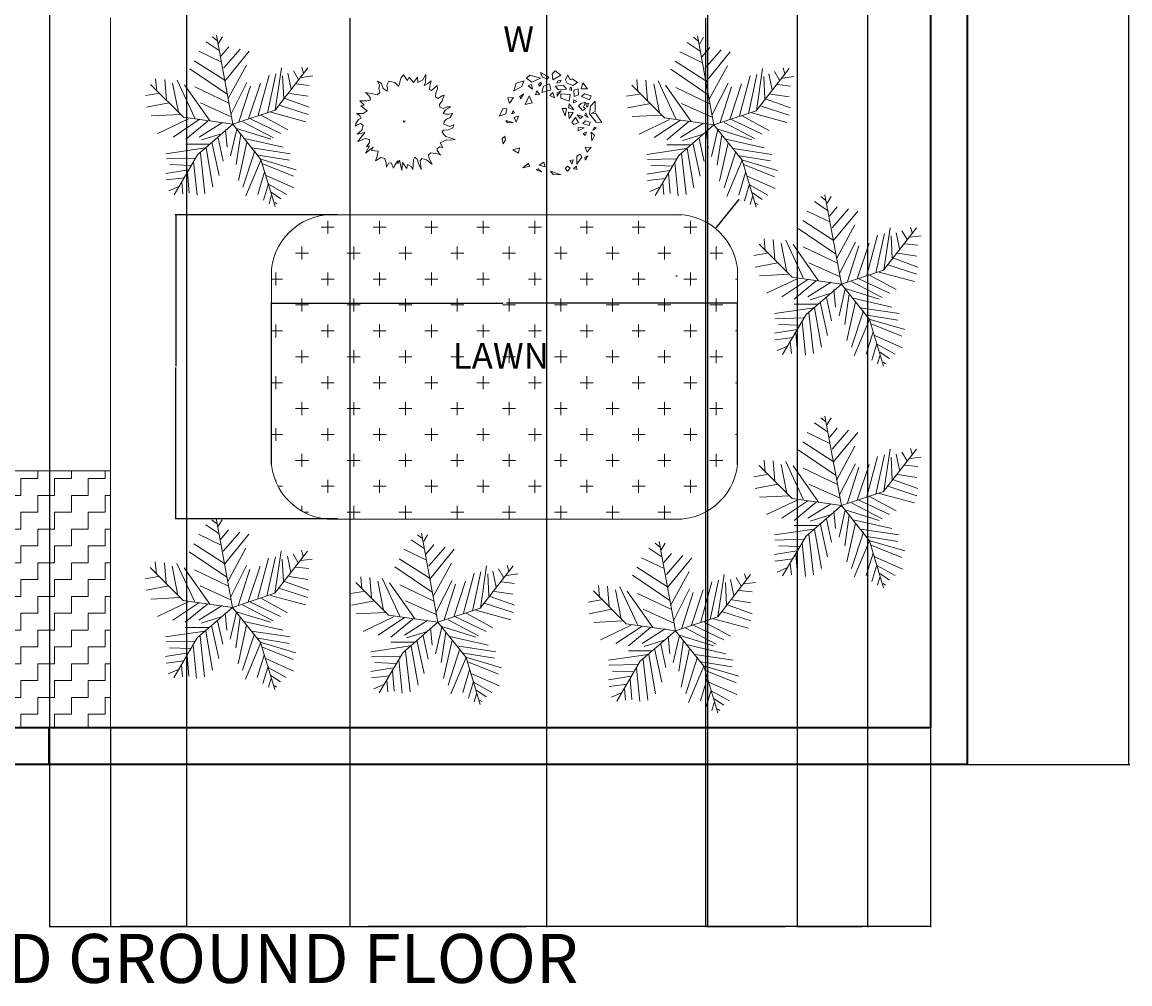
# Model space of a CAD drawing. Units: inches. Extents: x 2284 to 2815, y 1123 to 1948.
# Tile 3 of 6: x 2543 to 2814, y 1123 to 1358. Entities that reach past the tile are written whole.
import ezdxf

# ---------------------------------------------------------------- set-up
doc = ezdxf.new("R2010")
doc.units = ezdxf.units.IN
for name, color, linetype, lineweight in [('A-ANNO-DIMS', 2, 'Continuous', 18), ('A-ANNO-TITL', 30, 'Continuous', 35), ('A-AREA-IDEN', 30, 'Continuous', 18), ('A-WALL-PATT', 140, 'Continuous', 13), ('C-PVMT-PATT', 55, 'Continuous', 13), ('C-SITE-PVMT', 7, 'Continuous', 18), ('C-SITE-WALL', 7, 'Continuous', 35), ('L-FENC-GATE', 190, 'Continuous', 25), ('L-PLNT-BEDS', 90, 'Continuous', 18), ('L-PLNT-PATT', 40, 'Continuous', 13), ('TEXT', 30, 'Continuous', 18), ('TREE', 90, 'Continuous', 13)]:
    doc.layers.add(name, color=color, linetype=linetype, lineweight=lineweight)
doc.styles.get("Standard").update_dxf_attribs({"font": 'arial.ttf'})
doc.dimstyles.get("Standard").update_dxf_attribs({"dimtxt": 0.18, "dimasz": 0.18, "dimexe": 0.18, "dimexo": 0.0625, "dimgap": 0.09, "dimtad": 0, "dimtih": 1, "dimtoh": 1, "dimdec": 4, "dimzin": 0, "dimdsep": 46, "dimtxsty": 'Standard', "dimcen": 0.09, "dimadec": 0, "dimazin": 0, "dimtfac": 1, "dimtdec": 4, "dimtofl": 0, "dimtmove": 0, "dimatfit": 3, "dimfxl": 1, "dimtolj": 1, "dimtzin": 0, "dimarcsym": 0})

# ---------------------------------------------------------------- blocks, each defined once
blk = doc.blocks.new('*U9')
for points in [[(0, 60.64), (-3.051, 56.238), (-4.196, 52.815), (-5.34, 47.925), (-6.103, 45.969), (-11.062, 50.859), (-18.691, 52.326), (-20.98, 47.436), (-20.217, 43.524), (-20.598, 39.611), (-25.939, 43.035), (-27.846, 49.392), (-33.186, 52.326), (-30.516, 47.436), (-31.279, 43.035), (-30.135, 38.144), (-33.568, 35.21), (-40.815, 36.677), (-49.208, 38.144), (-46.919, 36.677), (-42.341, 31.787), (-42.341, 28.364), (-46.537, 27.386), (-55.692, 27.386), (-49.97, 22.006), (-54.548, 21.028), (-46.156, 14.671), (-51.496, 11.248), (-59.888, 11.248), (-55.692, 8.803), (-53.785, 5.38), (-57.218, 3.423), (-60.651, -1.467), (-61.033, -4.89), (-59.125, -3.423), (-54.548, -1.467), (-51.496, -4.401), (-53.022, -10.269), (-59.125, -15.16), (-49.208, -13.204), (-58.362, -24.451), (-48.445, -21.028), (-43.486, -22.495), (-43.104, -25.918), (-47.3, -31.298), (-43.104, -30.32), (-48.445, -39.611), (-38.527, -31.787), (-40.815, -36.188), (-32.423, -37.166), (-33.568, -43.523), (-35.475, -49.392), (-28.609, -44.99), (-23.65, -46.457), (-22.124, -51.837), (-21.743, -57.705), (-19.073, -52.326), (-15.639, -51.837), (-12.588, -58.683), (-11.062, -54.771), (-6.866, -49.392), (-6.866, -53.304), (-4.959, -48.414), (-1.907, -61.617), (-1.144, -51.348), (4.578, -59.172), (5.341, -54.282), (9.918, -56.727), (12.207, -60.639), (12.97, -47.925), (14.877, -44.501), (17.547, -47.436), (19.455, -52.815), (22.888, -60.639), (21.743, -49.392), (23.65, -46.457), (29.754, -47.925), (35.094, -52.326), (37.001, -53.793), (33.187, -46.457), (32.042, -41.567), (35.094, -39.122), (43.868, -40.589), (47.682, -42.056), (43.105, -36.188), (43.105, -33.743), (46.538, -31.298), (50.352, -32.765), (46.919, -26.407), (55.693, -22.495), (60.652, -22.984), (66.374, -22.006), (59.889, -20.05), (54.167, -18.094), (51.878, -15.649), (49.589, -12.225), (51.497, -10.269), (57.981, -9.78), (63.322, -7.335), (64.466, -2.934)], [(64.848, -2.934), (59.507, -5.379), (56.456, -4.401), (51.878, -2.445), (52.26, 0.978), (55.311, 3.912), (59.889, 5.869), (62.94, 11.248), (58.363, 10.27), (54.548, 10.27), (51.115, 11.248), (53.785, 15.649), (57.981, 18.094), (60.652, 19.561), (56.074, 19.561), (51.115, 17.605), (46.538, 19.072), (46.156, 22.496), (49.589, 27.386), (52.26, 34.721), (49.589, 33.743), (44.249, 30.32), (41.197, 32.276), (41.579, 37.655), (43.868, 42.546), (43.105, 46.947), (40.053, 44.013), (36.238, 40.589), (33.568, 42.057), (33.95, 45.969), (35.476, 52.815), (31.28, 49.392), (26.702, 46.947), (28.228, 50.859), (28.609, 61.129), (24.795, 54.282), (18.692, 50.859), (17.929, 57.706), (12.97, 50.859), (7.248, 57.706), (5.341, 53.304), (0, 60.64)]]:
    blk.add_lwpolyline(points)
blk.add_lwpolyline([(0.382, 1.956), (0, 0), (1.907, 0.489), (2.289, 1.467)], close=True)
blk = doc.blocks.new('*U6')
for p, q in [((0, 0), (-10.5, 57)), ((-8.737, 47.138), (-17.069, 52.711)), ((-10.186, 53.64), (-13.084, 55.962)), ((-9.099, 51.782), (-6.563, 55.962)), ((-7.288, 39.707), (-21.778, 46.673)), ((-7.65, 43.423), (-2.578, 49.46)), ((-5.839, 35.992), (4.667, 48.067)), ((-5.114, 27.632), (10.463, 46.673)), ((-3.665, 19.273), (-27.574, 35.527)), ((-5.114, 28.097), (-24.676, 40.636)), ((-2.941, 16.486), (8.652, 37.85)), ((27, 9), (48, 36)), ((27.127, 9.056), (31.112, 35.992)), ((44.153, 36.456), (45.239, 32.741)), ((-48.585, 21.131), (-49.309, 29.026)), ((-43.513, 28.561), (-42.427, 15.558)), ((16.259, 5.805), (23.142, 31.348)), ((22.055, 7.198), (27.489, 32.277)), ((31.836, 30.883), (32.561, 16.486)), ((35.096, 32.741), (37.27, 22.524)), ((38.719, 34.134), (41.979, 28.561)), ((43.791, 29.954), (51.036, 30.883)), ((-31.5, 4.5), (-52.5, 25.5)), ((-38.442, 26.239), (-34.819, 7.663)), ((-35.544, 28.097), (-24.314, 3.947)), ((-14.533, 2.09), (-30.834, 25.31)), ((-24.314, 23.917), (-2.941, 13.7)), ((-1.129, 6.734), (9.014, 26.704)), ((3.942, 1.625), (11.187, 24.381)), ((10.101, 3.483), (17.708, 26.239)), ((40.53, 25.775), (48.862, 24.846)), ((-47.498, 19.737), (-55.83, 18.344)), ((33.285, 16.486), (48.862, 10.913)), ((36.183, 19.737), (48.137, 17.88)), ((-40.615, 13.7), (-55.105, 10.913)), ((-20.691, 13.7), (-1.129, 4.876)), ((0, 0), (27, 9)), ((24.229, 7.663), (46.688, 1.625)), ((29.662, 12.307), (48.137, 6.269)), ((-33.37, 6.269), (-52.207, 5.34)), ((-28.299, 3.483), (-47.86, -5.805)), ((-21.416, 3.018), (-38.079, -8.128)), ((0, 0), (-31.5, 4.5)), ((-15.982, 2.09), (-30.11, -9.521)), ((0, 0), (-22.5, -19.5)), ((-6.563, 1.161), (-21.416, -8.128)), ((0, 0), (18, -22.5)), ((6.478, 1.625), (26.04, -8.592)), ((11.187, 3.483), (30.749, -5.805)), ((18.07, 5.805), (35.096, -3.483)), ((-6.563, -5.805), (-19.967, -9.985)), ((-4.752, -3.483), (-3.665, -14.629)), ((2.493, -3.019), (-1.491, -20.202)), ((1.769, -2.555), (24.229, -9.521)), ((5.029, -6.27), (2.131, -25.775)), ((-15.257, -12.772), (-30.11, -12.772)), ((-13.446, -11.378), (-8.737, -32.741)), ((-9.461, -8.592), (-6.201, -23.453)), ((9.014, -11.378), (3.58, -35.992)), ((7.565, -9.056), (32.198, -14.629)), ((-17.431, -15.094), (-42.789, -18.809)), ((-22.5, -19.5), (-37.5, -45)), ((-20.691, -18.345), (-17.793, -44.352)), ((-17.069, -15.094), (-12.721, -40.172)), ((14.085, -16.951), (6.478, -40.172)), ((12.274, -15.094), (36.907, -18.809)), ((16.259, -19.738), (36.183, -22.989)), ((-24.314, -21.596), (-42.427, -22.06)), ((-26.849, -26.24), (-40.253, -25.775)), ((-25.038, -23.918), (-22.865, -45.281)), ((18.07, -22.524), (8.289, -45.745)), ((18, -22.5), (27, -52.5)), ((18.433, -22.524), (40.53, -29.026)), ((19.157, -25.311), (38.719, -33.206)), ((-28.299, -29.026), (-42.789, -31.348)), ((-30.834, -34.135), (-42.427, -35.528)), ((-29.023, -30.884), (-27.936, -43.887)), ((20.244, -30.419), (15.897, -44.816)), ((21.331, -32.741), (39.081, -40.636)), ((-34.457, -39.708), (-40.978, -42.494)), ((-32.646, -36.921), (-31.921, -44.352)), ((22.78, -37.85), (19.519, -48.532)), ((22.78, -38.314), (34.372, -44.816)), ((24.591, -45.745), (23.142, -50.854)), ((24.591, -43.423), (30.749, -47.603)), ((26.764, -49.925), (28.213, -50.854))]:
    blk.add_line(p, q)
blk = doc.blocks.new('*U10')
for points in [[(-4.43, 11.05), (-5.18, 10.36), (-3.96, 9.49), (-2.07, 10.36)], [(-2, 11.66), (-1.6, 10.62), (-0.52, 10.1), (-0.18, 10.62), (-0.79, 10.96)], [(1.24, 12), (0.56, 11.31), (0.76, 10.01), (2.52, 11.05)], [(4.14, 11.14), (3.6, 10.01), (4, 9.23), (5.22, 8.71), (6.3, 9.41), (5.08, 10.19), (4.61, 10.01)], [(-5.78, 9.75), (-7.54, 9.23), (-8.01, 7.5), (-6.26, 8.45)], [(-4.84, 8.63), (-3.83, 7.85), (-4.03, 8.97)], [(-2.88, 7.5), (-3.15, 6.64), (-2.27, 6.72)], [(-1.94, 9.49), (-2.48, 8.97), (-2.27, 8.54), (-1.8, 9.06)], [(0.02, 9.06), (-1.33, 8.54), (-1.73, 7.16), (0.29, 7.76)], [(1.37, 8.54), (3.13, 8.8), (3.8, 7.85), (1.91, 7.76)], [(2.59, 9.93), (1.84, 9.75), (1.64, 9.23), (2.32, 9.41)], [(1.71, 6.29), (1.71, 7.07), (2.65, 7.5), (2.11, 6.9)], [(4.61, 8.28), (4.54, 7.76), (4.95, 7.59), (4.95, 8.28)], [(6.43, 7.94), (5.49, 7.68), (5.56, 6.21), (6.5, 6.64)], [(7.45, 9.32), (7.11, 7.94), (8.52, 7.94)], [(-8.14, 6.03), (-9.36, 5.95), (-9.02, 4.73)], [(-5.78, 6.81), (-6.66, 6.21), (-6.52, 5.69)], [(-4.57, 6.38), (-5.45, 4.47), (-3.89, 4.82)], [(0.76, 7.16), (0.09, 6.46), (1.1, 5.95)], [(2.52, 6.81), (2.52, 5.86), (4.41, 5.17), (4.61, 6.72)], [(5.49, 5.51), (5.42, 4.82), (6.16, 5.08)], [(8.12, 4.99), (7.11, 4.65), (6.5, 4.13), (7.38, 3.09), (8.12, 3.52), (7.65, 3.87)], [(7.85, 6.81), (7.18, 6.21), (9, 5.51), (9.33, 6.38)], [(10.28, 5.17), (9.2, 4.04), (9, 2.31), (10.48, 0.49), (11.76, 0.41), (10.35, 2.48), (9.33, 2.4), (10.28, 2.83)], [(-11.32, 1.79), (-9.83, 2.31), (-9.63, 3.44), (-10.44, 3.52)], [(-8.21, 3.09), (-8.48, 2.31), (-7.87, 2.57)], [(3.53, 1.88), (2.86, 3.52), (3.8, 3.52)], [(4.41, 4.56), (4.27, 3.7), (5.49, 3.26)], [(4.27, 2.74), (5.29, 2.66), (4.41, 1.27)], [(8.19, 2.57), (7.92, 2.05), (8.66, 1.53)], [(8.73, 4.73), (8.19, 4.56), (8.39, 3.87), (8.59, 4.04)], [(-8.21, 0.41), (-9.43, 0.32), (-9.83, 0.84)], [(-7, 1.79), (-7.94, 1.53), (-7.47, 0.49)], [(5.83, 1.53), (5.02, 0.41), (5.49, -0.02), (6.5, 0.41)], [(7.51, 1.71), (6.91, 1.27), (6.23, 2.14)], [(8.12, 0.75), (7.51, 0.15), (8.93, -0.28), (9.13, 0.49)], [(7.78, -0.8), (6.43, -1.5), (6.43, -0.72)], [(8.32, -1.75), (7.98, -2.53), (7.58, -2.1)], [(9.33, -1.75), (9.54, -3.74), (10.14, -2.53)], [(10.08, -0.63), (9.74, -1.32), (10.48, -0.89)], [(-10.03, -2.71), (-10.64, -3.31), (-10.44, -4.44), (-9.9, -3.49)], [(-8.28, -5.73), (-6.79, -5.3), (-7, -6.51)], [(6.1, -8.94), (6.16, -7.21), (6.91, -6.69), (7.24, -7.38)], [(8.05, -8.07), (8.59, -7.12), (7.92, -7.55)], [(9.33, -5.13), (8.46, -6.25), (7.98, -5.22)], [(-4.84, -8.85), (-4.43, -9.45), (-5.99, -9.8)], [(-2.34, -9.2), (-1.26, -8.5), (-0.99, -9.54)], [(4.07, -9.45), (3.53, -9.97), (4.07, -10.58), (4.61, -9.89)], [(5.29, -7.98), (4.61, -8.16), (5.02, -8.94)], [(6.03, -9.45), (5.42, -9.97), (6.16, -10.15)], [(-2.54, -10.06), (-3.02, -10.23), (-1.8, -10.67)], [(0.22, -10.58), (0.83, -11.27), (2.59, -11.36)]]:
    blk.add_lwpolyline(points, close=True)
blk = doc.blocks.new('*D21')
at = {"layer": 'A-ANNO-DIMS', "color": 0, "lineweight": -2, "transparency": 16777216}
for p, q in [((2774.62, 1908.4), (2814.43, 1908.4)), ((2814.25, 1908.22), (2814.25, 1542.59)), ((2814.25, 1176.58), (2814.25, 1542.22)), ((2774.62, 1176.4), (2814.43, 1176.4))]:
    blk.add_line(p, q, dxfattribs=at)
at = {"layer": 'A-ANNO-DIMS', "color": 0, "transparency": 16777216}
for points in [[(2814.22, 1908.22), (2814.28, 1908.22), (2814.25, 1908.4)], [(2814.22, 1176.58), (2814.28, 1176.58), (2814.25, 1176.4)]]:
    blk.add_solid(points, dxfattribs=at)
at = {"layer": 'Defpoints', "color": 0, "transparency": 16777216}
for p in [(2774.55, 1908.4), (2814.25, 1908.4), (2774.55, 1176.4)]:
    blk.add_point(p, dxfattribs=at)
at = {"layer": 'A-ANNO-DIMS', "color": 0, "transparency": 16777216, "insert": (2814.25, 1542.4), "char_height": 0.18, "attachment_point": 5}
blk.add_mtext('\\A1;732', dxfattribs=at)
blk = doc.blocks.new('*D41')
at = {"layer": 'A-ANNO-DIMS', "color": 0, "lineweight": -2, "transparency": 16777216}
for p, q in [((2564.55, 1185.34), (2564.55, 1136.52)), ((2765.55, 1185.34), (2765.55, 1136.52)), ((2564.73, 1136.7), (2664.78, 1136.7)), ((2765.37, 1136.7), (2665.33, 1136.7))]:
    blk.add_line(p, q, dxfattribs=at)
at = {"layer": 'A-ANNO-DIMS', "color": 0, "transparency": 16777216}
for points in [[(2564.73, 1136.73), (2564.73, 1136.67), (2564.55, 1136.7)], [(2765.37, 1136.73), (2765.37, 1136.67), (2765.55, 1136.7)]]:
    blk.add_solid(points, dxfattribs=at)
at = {"layer": 'Defpoints', "color": 0, "transparency": 16777216}
for p in [(2564.55, 1185.4), (2765.55, 1185.4), (2765.55, 1136.7)]:
    blk.add_point(p, dxfattribs=at)
at = {"layer": 'A-ANNO-DIMS', "color": 0, "transparency": 16777216, "insert": (2665.05, 1136.7), "char_height": 0.18, "attachment_point": 5}
blk.add_mtext('\\A1;201', dxfattribs=at)
blk = doc.blocks.new('*D42')
at = {"layer": 'A-ANNO-DIMS', "color": 0, "lineweight": -2, "transparency": 16777216}
for p, q in [((2623.18, 1359.34), (2623.18, 1136.52)), ((2710.41, 1359.34), (2710.41, 1136.52)), ((2623.36, 1136.7), (2666.4, 1136.7)), ((2710.23, 1136.7), (2667.19, 1136.7))]:
    blk.add_line(p, q, dxfattribs=at)
at = {"layer": 'A-ANNO-DIMS', "color": 0, "transparency": 16777216}
for points in [[(2623.36, 1136.73), (2623.36, 1136.67), (2623.18, 1136.7)], [(2710.23, 1136.73), (2710.23, 1136.67), (2710.41, 1136.7)]]:
    blk.add_solid(points, dxfattribs=at)
at = {"layer": 'Defpoints', "color": 0, "transparency": 16777216}
for p in [(2623.18, 1359.4), (2710.41, 1359.4), (2710.41, 1136.7)]:
    blk.add_point(p, dxfattribs=at)
at = {"layer": 'A-ANNO-DIMS', "color": 0, "transparency": 16777216, "insert": (2666.79, 1136.7), "char_height": 0.18, "attachment_point": 5}
blk.add_mtext('\\A1;87.23', dxfattribs=at)
blk = doc.blocks.new('*D44')
at = {"layer": 'A-ANNO-DIMS', "color": 0, "lineweight": -2, "transparency": 16777216}
for p, q in [((2583.19, 1836.34), (2583.19, 1136.52)), ((2671.4, 1836.34), (2671.4, 1136.52)), ((2583.37, 1136.7), (2626.92, 1136.7)), ((2671.22, 1136.7), (2627.67, 1136.7))]:
    blk.add_line(p, q, dxfattribs=at)
at = {"layer": 'A-ANNO-DIMS', "color": 0, "transparency": 16777216}
for points in [[(2583.37, 1136.73), (2583.37, 1136.67), (2583.19, 1136.7)], [(2671.22, 1136.73), (2671.22, 1136.67), (2671.4, 1136.7)]]:
    blk.add_solid(points, dxfattribs=at)
at = {"layer": 'Defpoints', "color": 0, "transparency": 16777216}
for p in [(2583.19, 1836.4), (2671.4, 1836.4), (2671.4, 1136.7)]:
    blk.add_point(p, dxfattribs=at)
at = {"layer": 'A-ANNO-DIMS', "color": 0, "transparency": 16777216, "insert": (2627.29, 1136.7), "char_height": 0.18, "attachment_point": 5}
blk.add_mtext('\\A1;88.21', dxfattribs=at)
blk = doc.blocks.new('*D45')
at = {"layer": 'A-ANNO-DIMS', "color": 0, "lineweight": -2, "transparency": 16777216}
for p, q in [((2549.55, 1836.34), (2549.55, 1136.52)), ((2583.19, 1836.34), (2583.19, 1136.52)), ((2549.73, 1136.7), (2565.91, 1136.7)), ((2583.01, 1136.7), (2566.84, 1136.7))]:
    blk.add_line(p, q, dxfattribs=at)
at = {"layer": 'A-ANNO-DIMS', "color": 0, "transparency": 16777216}
for points in [[(2549.73, 1136.73), (2549.73, 1136.67), (2549.55, 1136.7)], [(2583.01, 1136.73), (2583.01, 1136.67), (2583.19, 1136.7)]]:
    blk.add_solid(points, dxfattribs=at)
at = {"layer": 'Defpoints', "color": 0, "transparency": 16777216}
for p in [(2549.55, 1836.4), (2583.19, 1836.4), (2583.19, 1136.7)]:
    blk.add_point(p, dxfattribs=at)
at = {"layer": 'A-ANNO-DIMS', "color": 0, "transparency": 16777216, "insert": (2566.37, 1136.7), "char_height": 0.18, "attachment_point": 5}
blk.add_mtext('\\A1;33.635', dxfattribs=at)
blk = doc.blocks.new('*D49')
at = {"layer": 'A-ANNO-DIMS', "color": 0, "lineweight": -2, "transparency": 16777216}
for p, q in [((2732.88, 1524.34), (2732.88, 1136.52)), ((2765.55, 1524.34), (2765.55, 1136.52)), ((2733.06, 1136.7), (2748.82, 1136.7)), ((2765.37, 1136.7), (2749.61, 1136.7))]:
    blk.add_line(p, q, dxfattribs=at)
at = {"layer": 'A-ANNO-DIMS', "color": 0, "transparency": 16777216}
for points in [[(2733.06, 1136.73), (2733.06, 1136.67), (2732.88, 1136.7)], [(2765.37, 1136.73), (2765.37, 1136.67), (2765.55, 1136.7)]]:
    blk.add_solid(points, dxfattribs=at)
at = {"layer": 'Defpoints', "color": 0, "transparency": 16777216}
for p in [(2732.88, 1524.4), (2765.55, 1524.4), (2765.55, 1136.7)]:
    blk.add_point(p, dxfattribs=at)
at = {"layer": 'A-ANNO-DIMS', "color": 0, "transparency": 16777216, "insert": (2749.21, 1136.7), "char_height": 0.18, "attachment_point": 5}
blk.add_mtext('\\A1;32.68', dxfattribs=at)
blk = doc.blocks.new('*D51')
at = {"layer": 'A-ANNO-DIMS', "color": 0, "lineweight": -2, "transparency": 16777216}
for p, q in [((2710.87, 1388.93), (2710.87, 1136.52)), ((2750.11, 1388.93), (2750.11, 1136.52)), ((2711.05, 1136.7), (2730.03, 1136.7)), ((2749.93, 1136.7), (2730.95, 1136.7))]:
    blk.add_line(p, q, dxfattribs=at)
at = {"layer": 'A-ANNO-DIMS', "color": 0, "transparency": 16777216}
for points in [[(2711.05, 1136.73), (2711.05, 1136.67), (2710.87, 1136.7)], [(2749.93, 1136.73), (2749.93, 1136.67), (2750.11, 1136.7)]]:
    blk.add_solid(points, dxfattribs=at)
at = {"layer": 'Defpoints', "color": 0, "transparency": 16777216}
for p in [(2710.87, 1389), (2750.11, 1389), (2750.11, 1136.7)]:
    blk.add_point(p, dxfattribs=at)
at = {"layer": 'A-ANNO-DIMS', "color": 0, "transparency": 16777216, "insert": (2730.49, 1136.7), "char_height": 0.18, "attachment_point": 5}
blk.add_mtext('\\A1;39.234', dxfattribs=at)
blk = doc.blocks.new('*D57')
at = {"layer": 'A-ANNO-DIMS', "color": 0, "lineweight": -2, "transparency": 16777216}
for p, q in [((2604.02, 1249.87), (2604.02, 1289.69)), ((2604.2, 1289.51), (2660.68, 1289.51)), ((2718.06, 1289.51), (2661.59, 1289.51)), ((2718.24, 1249.87), (2718.24, 1289.69))]:
    blk.add_line(p, q, dxfattribs=at)
at = {"layer": 'A-ANNO-DIMS', "color": 0, "transparency": 16777216}
for points in [[(2604.2, 1289.54), (2604.2, 1289.48), (2604.02, 1289.51)], [(2718.06, 1289.54), (2718.06, 1289.48), (2718.24, 1289.51)]]:
    blk.add_solid(points, dxfattribs=at)
at = {"layer": 'Defpoints', "color": 0, "transparency": 16777216}
for p in [(2718.24, 1289.51), (2604.02, 1249.81), (2718.24, 1249.81)]:
    blk.add_point(p, dxfattribs=at)
at = {"layer": 'A-ANNO-DIMS', "color": 0, "transparency": 16777216, "insert": (2661.13, 1289.51), "char_height": 0.18, "attachment_point": 5}
blk.add_mtext('\\A1;114.22', dxfattribs=at)
blk = doc.blocks.new('*D58')
at = {"layer": 'A-ANNO-DIMS', "color": 0, "lineweight": -2, "transparency": 16777216}
for p, q in [((2620.16, 1311.15), (2580.34, 1311.15)), ((2580.52, 1310.97), (2580.52, 1274.05)), ((2580.52, 1236.77), (2580.52, 1273.69)), ((2620.16, 1236.59), (2580.34, 1236.59))]:
    blk.add_line(p, q, dxfattribs=at)
at = {"layer": 'A-ANNO-DIMS', "color": 0, "transparency": 16777216}
for points in [[(2580.49, 1310.97), (2580.55, 1310.97), (2580.52, 1311.15)], [(2580.49, 1236.77), (2580.55, 1236.77), (2580.52, 1236.59)]]:
    blk.add_solid(points, dxfattribs=at)
at = {"layer": 'Defpoints', "color": 0, "transparency": 16777216}
for p in [(2580.52, 1311.15), (2620.22, 1311.15), (2620.22, 1236.59)]:
    blk.add_point(p, dxfattribs=at)
at = {"layer": 'A-ANNO-DIMS', "color": 0, "transparency": 16777216, "insert": (2580.52, 1273.87), "char_height": 0.18, "attachment_point": 5}
blk.add_mtext('\\A1;74.56', dxfattribs=at)
blk = doc.blocks.new('*D59')
at = {"layer": 'A-ANNO-DIMS', "color": 0, "lineweight": -2, "transparency": 16777216}
for p, q in [((2718.52, 1314.79), (2712.94, 1307.96)), ((2718.7, 1314.79), (2718.52, 1314.79)), ((2703.25, 1296.21), (2703.43, 1296.21)), ((2703.34, 1296.12), (2703.34, 1296.3))]:
    blk.add_line(p, q, dxfattribs=at)
at = {"layer": 'A-ANNO-DIMS', "color": 0, "transparency": 16777216}
blk.add_solid([(2712.92, 1307.98), (2712.96, 1307.94), (2712.83, 1307.82)], dxfattribs=at)
at = {"layer": 'Defpoints', "color": 0, "transparency": 16777216}
for p in [(2712.83, 1307.82), (2703.34, 1296.21)]:
    blk.add_point(p, dxfattribs=at)
at = {"layer": 'A-ANNO-DIMS', "color": 0, "transparency": 16777216, "insert": (2719.44, 1314.79), "char_height": 0.18, "attachment_point": 5}
blk.add_mtext('\\A1;4X R14.997', dxfattribs=at)

msp = doc.modelspace()

# ---------------------------------------------------------------- hatches: boundary and pattern name
at = {"layer": 'A-WALL-PATT'}
h = msp.add_hatch(dxfattribs=at)
h.set_pattern_fill('AR-SAND', color=256, scale=8.5)
h.paths.add_polyline_path([(2339.554, 1899.404), (2375.554, 1899.404), (2765.554, 1899.404), (2765.554, 1185.404), (2549.3222, 1185.404), (2549.3222, 1176.404), (2774.554, 1176.404), (2774.554, 1908.404), (2330.554, 1908.404), (2330.554, 1176.404), (2349.4276, 1176.404), (2349.4276, 1185.404), (2339.554, 1185.404)])
h.paths.add_polyline_path([(2710.054, 1899.404), (2701.054, 1899.404), (2701.054, 1889.8374), (2710.054, 1889.8374)], flags=17)
at = {"layer": 'C-PVMT-PATT'}
h = msp.add_hatch(dxfattribs=at)
h.set_pattern_fill('ZIGZAG', color=256, scale=1.3)
h.set_pattern_definition([(0, (0, 0), (4.1275, 4.1275), [4.1275, -4.1275]), (90, (4.1275, 0), (-4.1275, 4.1275), [4.1275, -4.1275])])
h.paths.add_polyline_path([(2564.554, 1248.417), (2339.554, 1248.417), (2339.554, 1185.404), (2564.554, 1185.404)])
at = {"layer": 'L-PLNT-PATT'}
h = msp.add_hatch(dxfattribs=at)
h.set_pattern_fill('CROSS', color=256)
h.paths.add_polyline_path([(2718.2406, 1297.9246, 0.35632969), (2704.6415, 1311.1466), (2617.6203, 1311.1466, 0.35632969), (2604.0213, 1297.9246), (2604.0213, 1249.8094, 0.35632969), (2617.6203, 1236.5875), (2704.6415, 1236.5875, 0.35632969), (2718.2406, 1249.8094)])

# ---------------------------------------------------------------- linework, layer by layer
at = {"layer": 'C-SITE-PVMT'}
for p, q in [((2564.554, 1359.404), (2564.554, 1185.404)), ((2339.554, 1248.417), (2564.554, 1248.417))]:
    msp.add_line(p, q, dxfattribs=at)
at = {"layer": 'C-SITE-WALL'}
for p, q in [((2774.554, 1908.404), (2774.554, 1176.404)), ((2765.554, 1899.404), (2765.554, 1185.404)), ((2765.554, 1185.404), (2339.554, 1185.404)), ((2774.554, 1176.404), (2330.554, 1176.404))]:
    msp.add_line(p, q, dxfattribs=at)
at = {"layer": 'L-FENC-GATE'}
msp.add_line((2549.3222, 1185.404), (2549.3222, 1176.404), dxfattribs=at)
at = {"layer": 'L-PLNT-BEDS'}
for points in [[(2617.6203, 1311.1466), (2704.6415, 1311.1466)], [(2604.0213, 1249.8094), (2604.0213, 1297.9246)], [(2718.2406, 1297.9246), (2718.2406, 1249.8094)], [(2704.6415, 1236.5875), (2617.6203, 1236.5875)]]:
    msp.add_lwpolyline(points, dxfattribs=at)
for centre, start, end in [((2618.9194, 1296.206), 85.030532, 173.41944), ((2703.3424, 1296.206), 6.58056, 94.969468), ((2618.9194, 1251.5281), 186.58056, 274.969468), ((2703.3424, 1251.5281), 265.030532, 353.41944)]:
    msp.add_arc(centre, 14.997, start, end, dxfattribs=at)

# ---------------------------------------------------------------- block references
at = {"layer": 'TREE'}
for name, p, xscale, yscale, zscale in [('*U6', (2594.5131, 1333.3351), 0.383737482457664, 0.383737482457664, 0.383737482457664), ('*U6', (2712.4723, 1333.1807), 0.383737482457664, 0.383737482457664, 0.383737482457664), ('*U9', (2636.3223, 1333.8468), 0.1916033270346016, 0.1916033270346016, 0.1916033270346016), ('*U10', (2672.1718, 1333.3502), 1.090243299178313, 1.090243299178313, 1.090243299178313), ('*U6', (2743.717, 1294.1583), 0.383737482457664, 0.383737482457664, 0.383737482457664), ('*U6', (2743.717, 1239.8986), 0.383737482457664, 0.383737482457664, 0.383737482457664), ('*U6', (2594.4185, 1214.9223), 0.383737482457664, 0.383737482457664, 0.383737482457664), ('*U6', (2644.7991, 1211.269), 0.383737482457664, 0.383737482457664, 0.383737482457664), ('*U6', (2703.0656, 1209.19), 0.383737482457664, 0.383737482457664, 0.383737482457664)]:
    msp.add_blockref(name, p, dxfattribs=dict(at, xscale=xscale, yscale=yscale, zscale=zscale))

# ---------------------------------------------------------------- texts
at = {"layer": 'A-ANNO-TITL', "insert": (2464.2261, 1134.8759), "char_height": 12.014871, "attachment_point": 1}
msp.add_mtext_dynamic_manual_height_columns('PROPOSED GROUND FLOOR', width=350.083049, gutter_width=60.0744, heights=[0], dxfattribs=at)
at = {"layer": 'A-AREA-IDEN', "insert": (2648.4133, 1279.7088), "char_height": 6.28983, "attachment_point": 1}
msp.add_mtext_dynamic_manual_height_columns('LAWN', width=114.078767, gutter_width=31.4491, heights=[0], dxfattribs=at)
at = {"layer": 'TEXT', "insert": (2660.8134, 1357.3427), "char_height": 6.2898, "attachment_point": 1}
msp.add_mtext_dynamic_manual_height_columns('W', width=114.078767, gutter_width=31.4491, heights=[0], dxfattribs=at)

# ---------------------------------------------------------------- dimensions: what is measured, and where the dimension line sits
at = {"layer": 'A-ANNO-DIMS'}
for base, p1, p2, override, picture, middle in [((2814.254, 1908.404), (2774.554, 1176.404), (2774.554, 1908.404), {"dimdec": 0, "dimlfac": 1, "dimrnd": 0, "dimzin": 0, "dimdsep": 46, "dimlunit": 2}, '*D21', (2814.254, 1542.404)), ((2580.5186, 1311.1466), (2620.2186, 1236.5875), (2620.2186, 1311.1466), {"dimdec": 2, "dimlfac": 1, "dimrnd": 0, "dimzin": 0, "dimdsep": 46, "dimlunit": 2}, '*D58', (2580.5186, 1273.867))]:
    dim = msp.add_linear_dim(base=base, p1=p1, p2=p2, angle=90, dimstyle='Standard', override=override, dxfattribs=at)
    dim.commit()
    dim.dimension.update_dxf_attribs({"geometry": picture, "text_midpoint": middle})
for base, p1, p2, override, picture, middle in [((2583.189, 1136.704), (2549.554, 1836.404), (2583.189, 1836.404), {"dimdec": 3, "dimlfac": 1, "dimrnd": 0, "dimzin": 0, "dimdsep": 46, "dimlunit": 2}, '*D45', (2566.3715, 1136.704)), ((2671.4007, 1136.704), (2583.189, 1836.404), (2671.4007, 1836.404), {"dimdec": 2, "dimlfac": 1, "dimrnd": 0, "dimzin": 0, "dimdsep": 46, "dimlunit": 2}, '*D44', (2627.2949, 1136.704)), ((2765.554, 1136.704), (2732.876, 1524.404), (2765.554, 1524.404), {"dimdec": 2, "dimlfac": 1, "dimrnd": 0, "dimzin": 0, "dimdsep": 46, "dimlunit": 2}, '*D49', (2749.215, 1136.704)), ((2750.1064, 1136.704), (2710.8724, 1388.9955), (2750.1064, 1388.9955), {"dimdec": 3, "dimlfac": 1, "dimrnd": 0, "dimzin": 0, "dimdsep": 46, "dimlunit": 2}, '*D51', (2730.4894, 1136.704)), ((2710.406, 1136.704), (2623.1768, 1359.404), (2710.406, 1359.404), {"dimdec": 2, "dimlfac": 1, "dimrnd": 0, "dimzin": 0, "dimdsep": 46, "dimlunit": 2}, '*D42', (2666.7914, 1136.704)), ((2718.2406, 1289.5094), (2604.0213, 1249.8094), (2718.2406, 1249.8094), {"dimdec": 2, "dimlfac": 1, "dimrnd": 0, "dimzin": 0, "dimdsep": 46, "dimlunit": 2}, '*D57', (2661.1309, 1289.5094)), ((2765.554, 1136.704), (2564.554, 1185.404), (2765.554, 1185.404), {"dimdec": 0, "dimlfac": 1, "dimrnd": 0, "dimzin": 0, "dimdsep": 46, "dimlunit": 2}, '*D41', (2665.054, 1136.704))]:
    dim = msp.add_linear_dim(base=base, p1=p1, p2=p2, dimstyle='Standard', override=override, dxfattribs=at)
    dim.commit()
    dim.dimension.update_dxf_attribs({"geometry": picture, "text_midpoint": middle})
dim = msp.add_radius_dim(center=(2703.3424, 1296.206), mpoint=(2712.8258, 1307.8238), text='4X <>', dimstyle='Standard', override={"dimdec": 3, "dimlfac": 1, "dimrnd": 0, "dimzin": 0, "dimdsep": 46, "dimlunit": 2}, dxfattribs=at)
dim.commit()
dim.dimension.update_dxf_attribs({"geometry": '*D59', "text_midpoint": (2719.4427, 1314.7945), "dimtype": 164})

doc.saveas('drawing.dxf')
